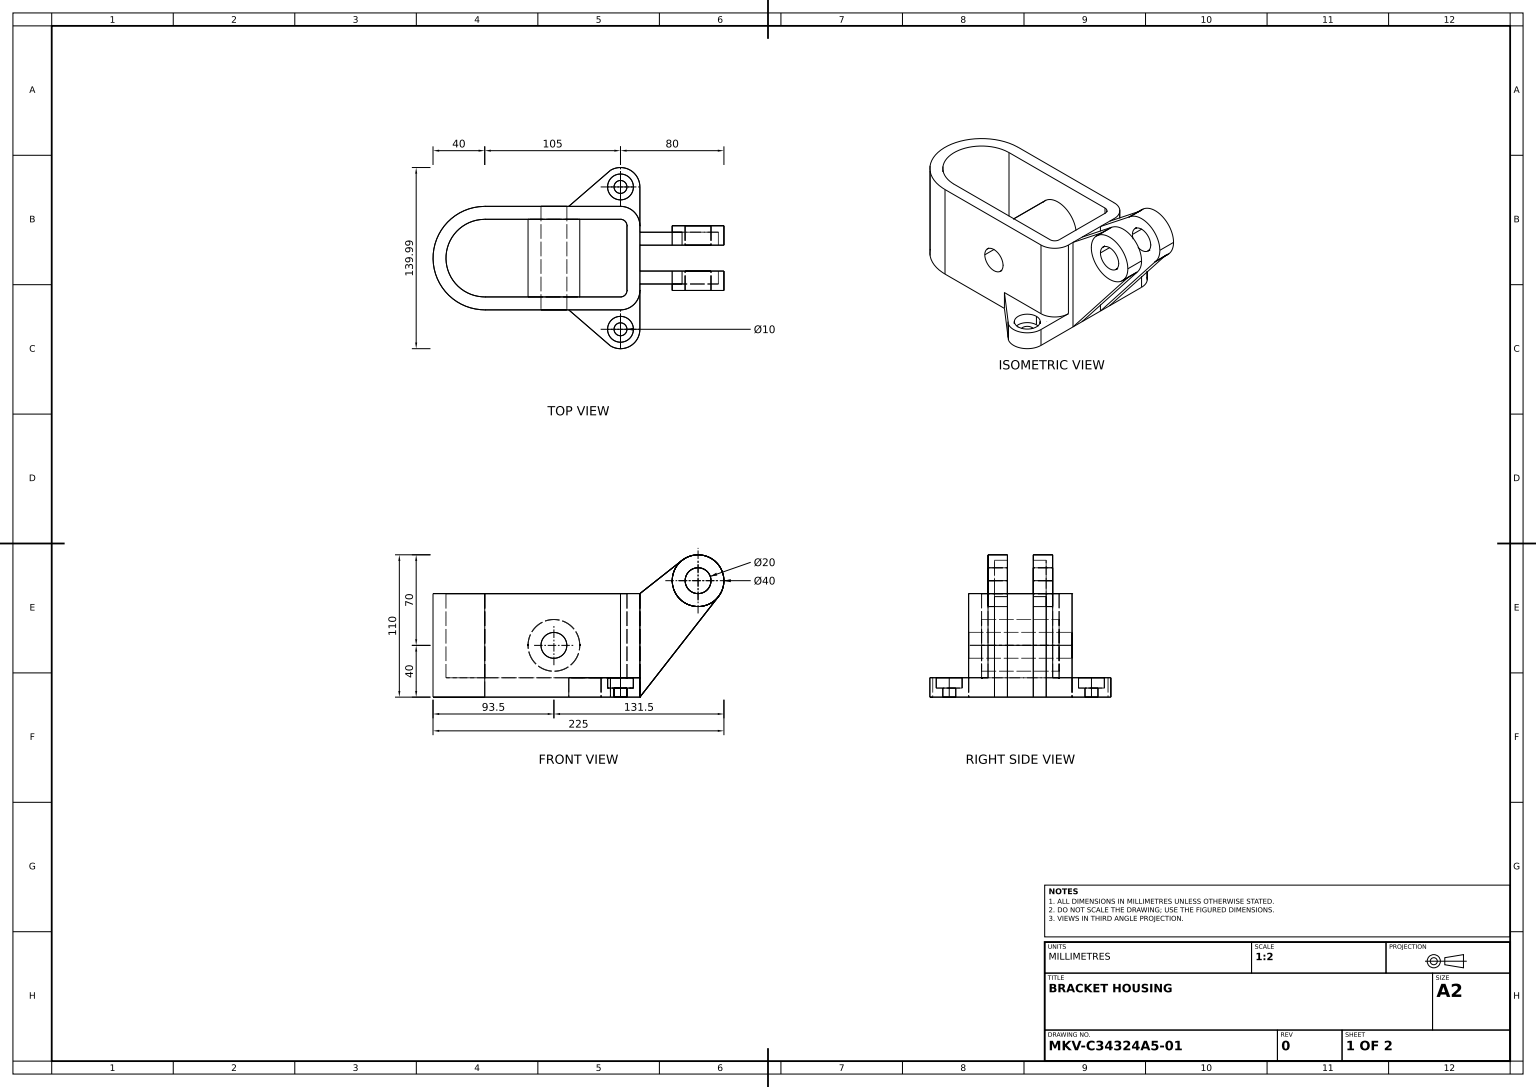
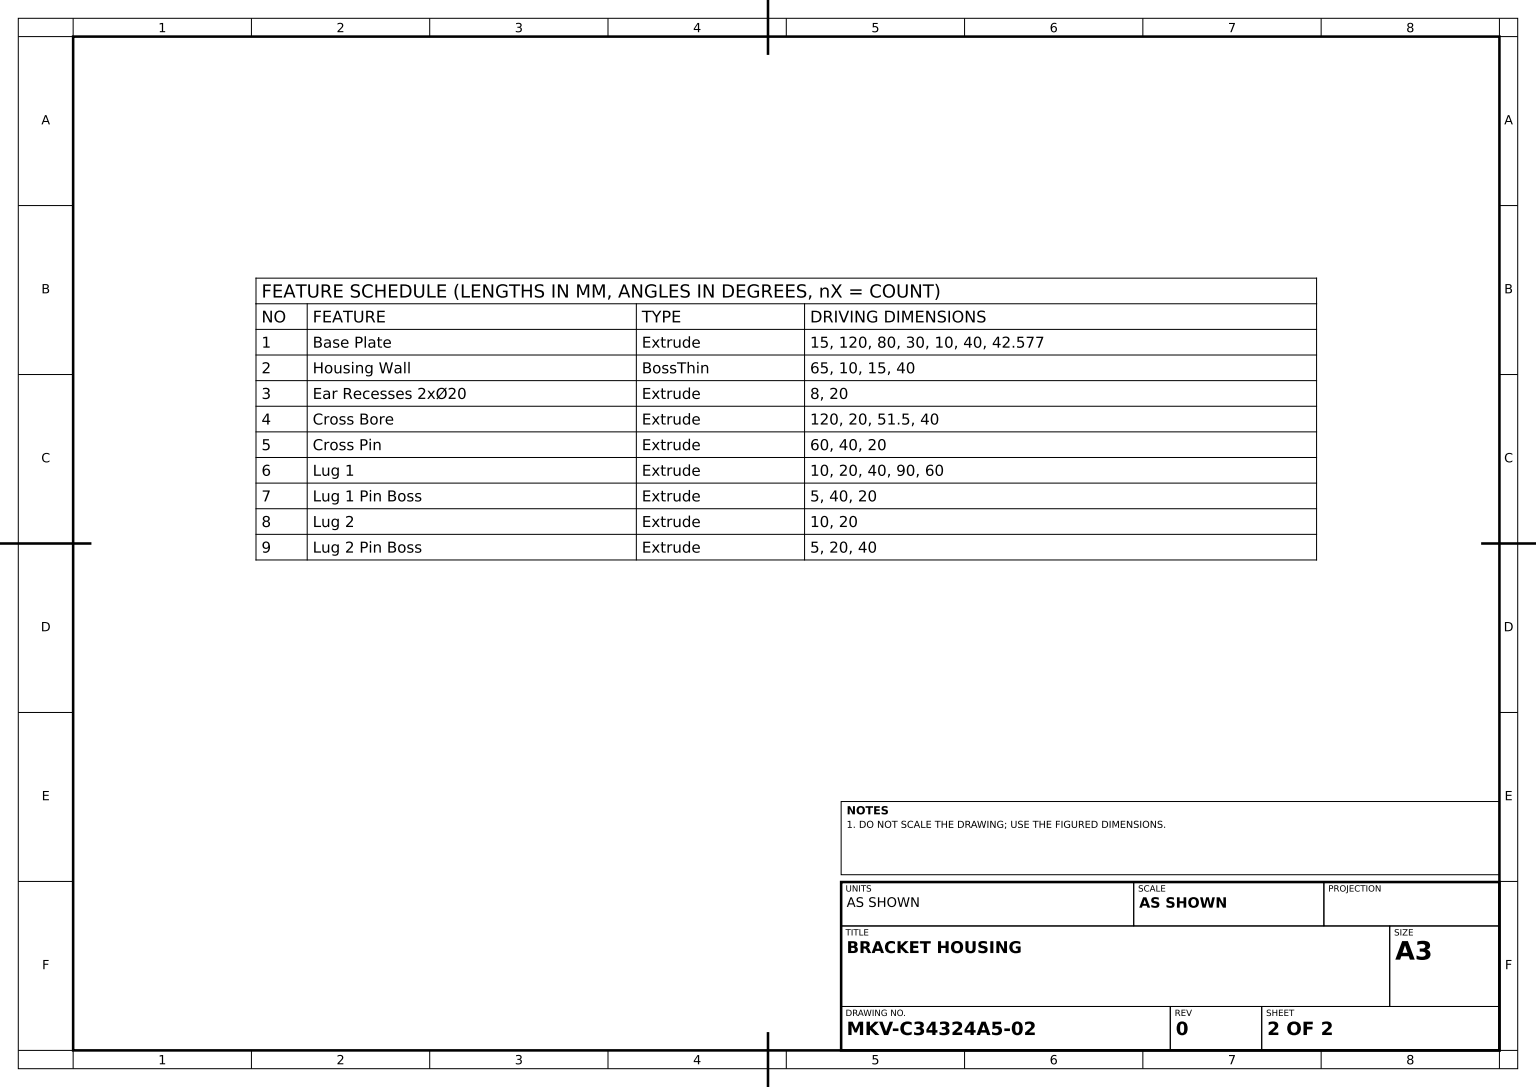
from build123d import *

# Parameters (mm, degrees)
BASE_PLATE_SKETCH_R       = 5
BASE_PLATE_DEPTH          = 15
HOUSING_WALL_DEPTH        = 65
EAR_RECESSES_SKETCH_R     = 10
EAR_RECESSES_2X_20_DEPTH  = 8
CROSS_BORE_SKETCH_R       = 10
CROSS_BORE_DEPTH          = 120
CROSS_START               = 60
CROSS_PIN_SKETCH_R        = 20
CROSS_PIN_SKETCH_R_2      = 10
CROSS_PIN_DEPTH           = 60
LUG_1_SKETCH_R            = 20
LUG_1_SKETCH_R_2          = 10
LUG_1_DEPTH               = 10
LUG_1_PIN_BOSS_SKETCH_R   = 20
LUG_1_PIN_BOSS_SKETCH_R_2 = 10
LUG_1_PIN_BOSS_DEPTH      = 5
LUG_START                 = -10
LUG_2_SKETCH_R            = 20
LUG_2_SKETCH_R_2          = 10
LUG_2_DEPTH               = 10
LUG_START_2               = 5
LUG_2_PIN_BOSS_SKETCH_R   = 20
LUG_2_PIN_BOSS_SKETCH_R_2 = 10
LUG_2_PIN_BOSS_DEPTH      = 5


with BuildPart() as part:
    # Base Plate Sketch → Base Plate (new body)
    # profile 1 of 3: a face of its own
    with BuildSketch(Plane(origin=(0, 0, 0), x_dir=(1, 0, 0), z_dir=(0, 1, 0))):
        with BuildLine():
            Line((-60, -40), (45, -40))
            ThreePointArc((45, -40), (55.606601718, -35.606601718), (60, -25))
            Line((60, -25), (60, 25))
            ThreePointArc((60, 25), (55.606601718, 35.606601718), (45, 40))
            Line((45, 40), (-60, 40))
            ThreePointArc((-60, 40), (-100, 0), (-60, -40))
        make_face()
    # profile 2 of 3: a face of its own
    with BuildSketch(Plane(origin=(0, 0, 0), x_dir=(1, 0, 0), z_dir=(0, 1, 0))):
        with BuildLine():
            Line((60, -40), (60, -25))
            ThreePointArc((60, -25), (55.606601718, -35.606601718), (45, -40))
            Line((45, -40), (5, -40))
            Line((5, -40), (33.441882385, -64.560853371))
            Line((33.441882385, -64.560853371), (37.224740847, -67.827522953))
            ThreePointArc((37.224740847, -67.827522953), (52.361083912, -68.06959998), (60, -55))
            Line((60, -55), (60, -40))
        make_face()
        with Locations(Location((45, -55, 0), (0, 0, 270))):
            Circle(BASE_PLATE_SKETCH_R, mode=Mode.SUBTRACT)
    # profile 3 of 3: a face of its own
    with BuildSketch(Plane(origin=(0, 0, 0), x_dir=(1, 0, 0), z_dir=(0, 1, 0))):
        with BuildLine():
            Line((60, 40), (60, 55))
            ThreePointArc((60, 55), (52.361083912, 68.06959998), (37.224740847, 67.827522953))
            Line((37.224740847, 67.827522953), (33.441882385, 64.560853371))
            Line((33.441882385, 64.560853371), (5, 40))
            Line((5, 40), (45, 40))
            ThreePointArc((45, 40), (55.606601718, 35.606601718), (60, 25))
            Line((60, 25), (60, 40))
        make_face()
        with Locations(Location((45, 55, 0), (0, 0, 270))):
            Circle(BASE_PLATE_SKETCH_R, mode=Mode.SUBTRACT)
    extrude(amount=BASE_PLATE_DEPTH)

    # Housing Wall Sketch → Housing Wall (add)
    with BuildSketch(Plane(origin=(0, 15, 0), x_dir=(1, 0, 0), z_dir=(0, 1, 0))):
        with BuildLine():
            Line((45, 40), (-60, 40))
            ThreePointArc((-60, 40), (-100, 0), (-60, -40))
            Line((-60, -40), (45, -40))
            ThreePointArc((45, -40), (55.606601718, -35.606601718), (60, -25))
            Line((60, -25), (60, 25))
            ThreePointArc((60, 25), (55.606601718, 35.606601718), (45, 40))
        make_face()
        with BuildLine():
            Line((45, 30), (-60, 30))
            ThreePointArc((-60, 30), (-90, 0), (-60, -30))
            Line((-60, -30), (45, -30))
            ThreePointArc((45, -30), (48.535533906, -28.535533906), (50, -25))
            Line((50, -25), (50, 25))
            ThreePointArc((50, 25), (48.535533906, 28.535533906), (45, 30))
        make_face(mode=Mode.SUBTRACT)
    extrude(amount=HOUSING_WALL_DEPTH)

    # Ear Recesses Sketch → Ear Recesses 2xØ20 (cut)
    with BuildSketch(Plane(origin=(0, 15, 0), x_dir=(1, 0, 0), z_dir=(0, 1, 0))):
        with Locations(Location((45, -55, 0), (0, 0, 270))):
            Circle(EAR_RECESSES_SKETCH_R)
        with Locations(Location((45, 55, 0), (0, 0, 270))):
            Circle(EAR_RECESSES_SKETCH_R)
    extrude(amount=-EAR_RECESSES_2X_20_DEPTH, mode=Mode.SUBTRACT)

    # Cross Bore Sketch → Cross Bore (cut)
    with BuildSketch(Plane.XY.offset(40)):
        with Locations((-6.5, 40)):
            Circle(CROSS_BORE_SKETCH_R)
    extrude(amount=-CROSS_BORE_DEPTH, mode=Mode.SUBTRACT)

    # Cross Pin Sketch → Cross Pin (add)
    with BuildSketch(Plane.XY.offset(-30).offset(CROSS_START)):
        with Locations((-6.5, 40)):
            Circle(CROSS_PIN_SKETCH_R)
        with Locations((-6.5, 40)):
            Circle(CROSS_PIN_SKETCH_R_2, mode=Mode.SUBTRACT)
    extrude(amount=-CROSS_PIN_DEPTH)

    # Lug 1 Sketch → Lug 1 (add)
    # profile 1 of 2: a face of its own
    with BuildSketch(Plane.XY.offset(10)):
        with BuildLine():
            Line((92.6204123, 105.708144651), (60, 80))
            Line((60, 80), (60, 0))
            Line((60, 0), (120.753851487, 77.678629812))
            ThreePointArc((120.753851487, 77.678629812), (90.884057256, 75.831719919), (92.6204123, 105.708144651))
        make_face()
    # profile 2 of 2: a face of its own
    with BuildSketch(Plane.XY.offset(10)):
        with Locations((105, 90)):
            Circle(LUG_1_SKETCH_R)
        with Locations((105, 90)):
            Circle(LUG_1_SKETCH_R_2, mode=Mode.SUBTRACT)
    extrude(amount=LUG_1_DEPTH)

    # Lug 1 Pin Boss Sketch → Lug 1 Pin Boss (add)
    with BuildSketch(Plane.XY.offset(20)):
        with Locations(Location((105, 90, 0), (0, 0, 128.241642007))):
            Circle(LUG_1_PIN_BOSS_SKETCH_R)
        with Locations((105, 90)):
            Circle(LUG_1_PIN_BOSS_SKETCH_R_2, mode=Mode.SUBTRACT)
    extrude(amount=LUG_1_PIN_BOSS_DEPTH)

    # Lug 2 Sketch → Lug 2 (add)
    # profile 1 of 2: a face of its own
    with BuildSketch(Plane.XY.offset(-10).offset(LUG_START)):
        with BuildLine():
            ThreePointArc((120.753851487, 77.678629812), (90.884057256, 75.831719919), (92.6204123, 105.708144651))
            Line((92.6204123, 105.708144651), (60, 80))
            Line((60, 80), (60, 0))
            Line((60, 0), (120.753851487, 77.678629812))
        make_face()
    # profile 2 of 2: a face of its own
    with BuildSketch(Plane.XY.offset(-10).offset(LUG_START)):
        with Locations(Location((105, 90, 0), (0, 0, 128.241642007))):
            Circle(LUG_2_SKETCH_R)
        with Locations((105, 90)):
            Circle(LUG_2_SKETCH_R_2, mode=Mode.SUBTRACT)
    extrude(amount=LUG_2_DEPTH)

    # Lug 2 Pin Boss Sketch → Lug 2 Pin Boss (add)
    with BuildSketch(Plane(origin=(0, 0, -20), x_dir=(-1, 0, 0), z_dir=(0, 0, -1)).offset(LUG_START_2)):
        with Locations(Location((-105, 90, 0), (0, 0, 51.758357993))):
            Circle(LUG_2_PIN_BOSS_SKETCH_R)
        with Locations(Location((-105, 90, 0), (0, 0, 180))):
            Circle(LUG_2_PIN_BOSS_SKETCH_R_2, mode=Mode.SUBTRACT)
    extrude(amount=-LUG_2_PIN_BOSS_DEPTH)


solid = part.part
